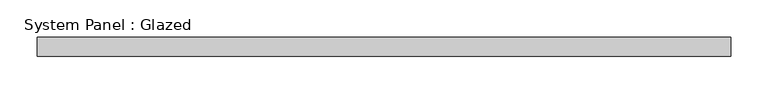
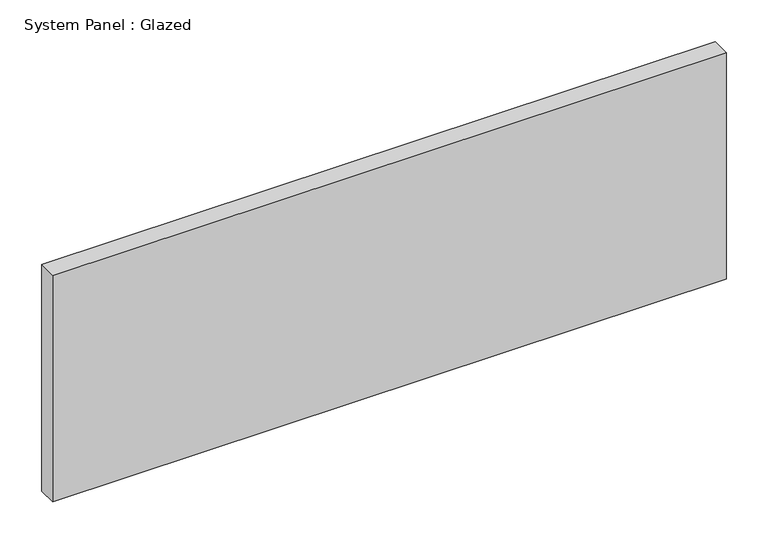
"""IFC4 building model written with IfcOpenShell, lengths in millimetres: plate geometry, System Panel : Glazed."""

from ifc_helpers import new_model, si_unit, origin, origin_with_axes, place, context, project, spatial, polyline, outline, extrude, source, transform, mapped, element, save


def system_panel_glazed_95b6fecb(model_context):
    return source(origin(), model_context, "Body", "SweptSolid", [
        extrude(outline(polyline([(463.5500002, 19.05), (-463.5500002, 19.05), (-463.5500002, 44.45), (463.5500002, 44.45), (463.5500002, 19.05)])), origin_with_axes(), (0.0, 0.0, 1.0), 330.2),
    ])


if __name__ == "__main__":
    model = new_model("IFC4")
    model_context = context("Model", 3, world=origin())
    ifc_project = project(units=[si_unit("LENGTHUNIT", "METRE", prefix="MILLI")], contexts=[model_context])
    site = spatial("IfcSite", under=ifc_project)
    building = spatial("IfcBuilding", under=site)
    placement = place(None, origin())
    system_panel_glazed_shape = system_panel_glazed_95b6fecb(model_context)
    element("IfcPlate", 1, ObjectType="System Panel : Glazed", at=placement, inside=building, context=model_context, shape_type="MappedRepresentation", body=[
        mapped(system_panel_glazed_shape, transform((0.0, 0.0, 0.0), x_axis=(1.0, 0.0, 0.0), y_axis=(0.0, 1.0, 0.0), z_axis=(0.0, 0.0, 1.0))),
    ])
    save(model, "model.ifc")

# Revit data of these elements
# Type "System Panel : Glazed"
#   Construction Type Id = "GSP4R"
#   Analytic Construction = "1/8 in Pilkington single glazing"
#   Visual Light Transmittance = 0.9
#   Solar Heat Gain Coefficient = 0.86
#   Heat Transfer Coefficient (U) = 1.18115 BTU/(h·ft²·°F)
#   Define Thermal Properties by = 1
# Element 1 (IfcPlate, "System Panel : Glazed")
#   Materials on its faces: "Glass"
# Materials
#   "Glass": class "Glass", colour RGB 0 128 192, transparency 0.75, Description = "Soda Lime Glass", Cost = 0
